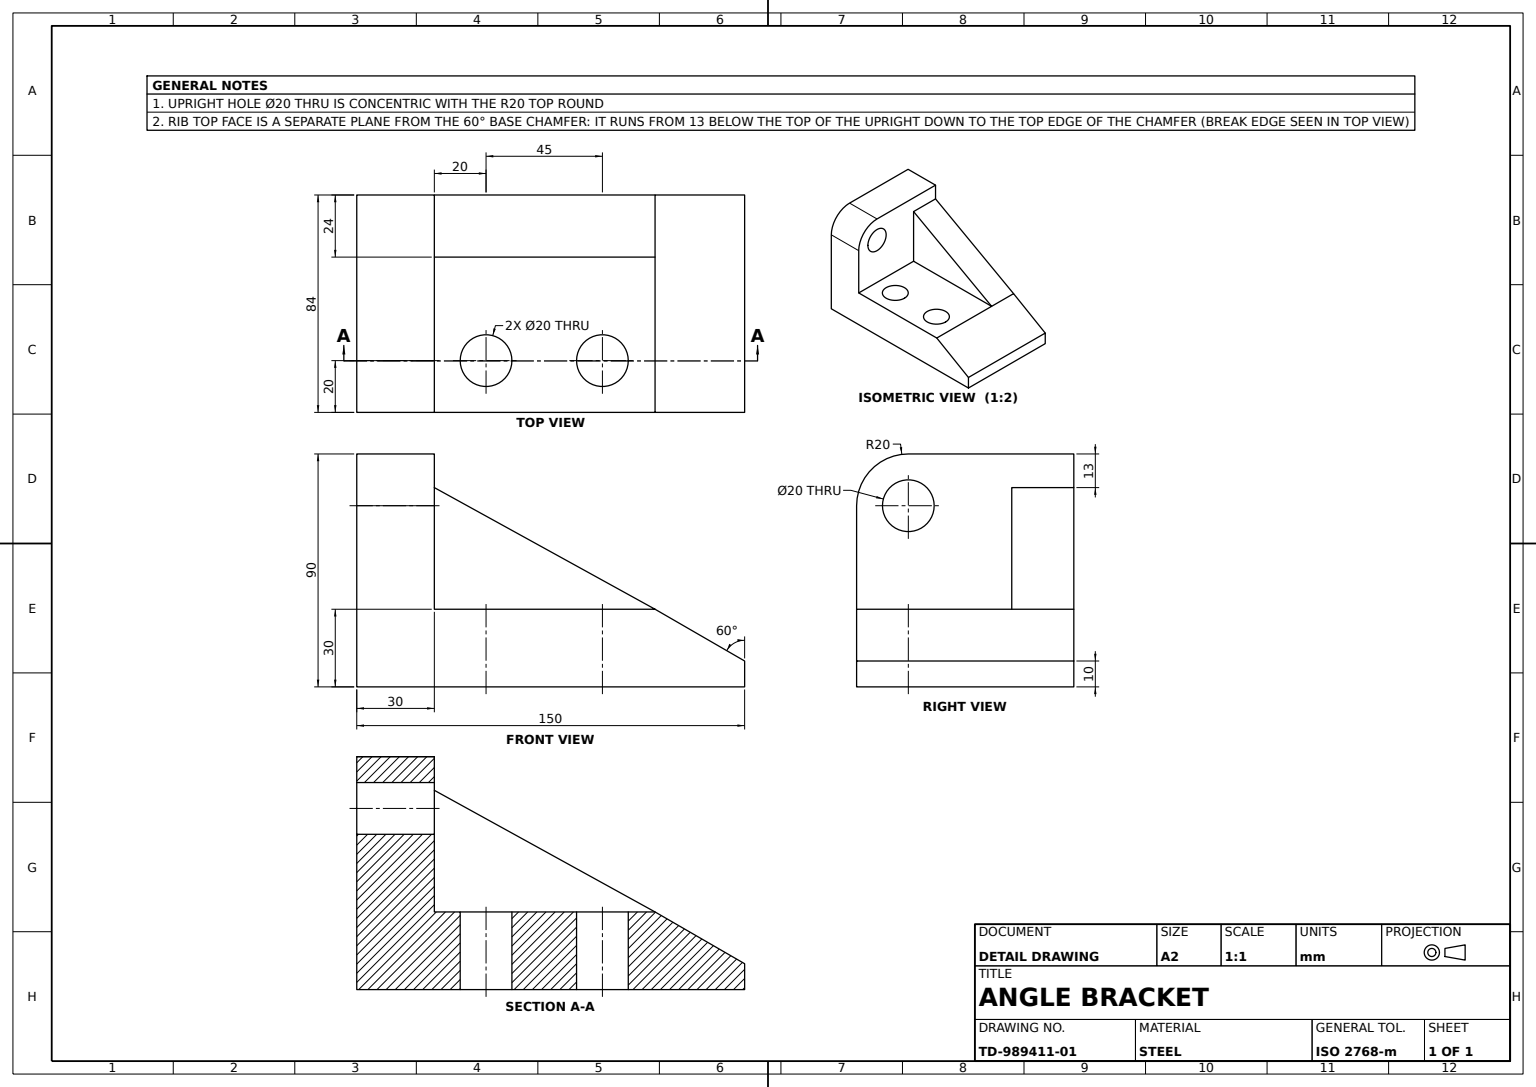
SolidWorks part; units mm, degrees
material "Plain Carbon Steel"
ref_plane "Front Plane" through (0, 0, 0) normal (0, 0, 1) x (1, 0, 0)
ref_plane "Top Plane" through (0, 0, 0) normal (0, 1, 0) x (1, 0, 0)
ref_plane "Right Plane" through (0, 0, 0) normal (1, 0, 0) x (0, 0, -1)
sketch "Bracket Profile Sketch" plane through (0, 0, 0) normal (0, 0, 1) x (1, 0, 0)
  line L0 (-75, 90) -> (-75, 0)
  line L1 (-75, 0) -> (75, 0)
  line L2 (75, 0) -> (75, 10)
  line L3 (75, 10) -> (40.359, 30)
  line L4 (40.359, 30) -> (-45, 30)
  line L5 (-45, 30) -> (-45, 90)
  line L6 (-45, 90) -> (-75, 90)
  dimension "D1" = 90
  dimension "D2" = 150
  dimension "D3" = 10
  dimension "D4" = 30
  dimension "D5" = 60
  dimension "D6" = 30
extrude "Bracket Body" add sketch "Bracket Profile Sketch" along normal mid plane 84
fillet "Upright Top Round R20" radius 20 1 edges at (-60, 90, 42)
sketch "Support Rib Sketch" plane through (0, 0, -42) normal (0, 0, -1) x (-1, 0, 0)
  line L0 (-40.359, 30) -> (45, 77)
  line L1 (45, 30) -> (45, 90) construction
  line L2 (45, 90) -> (75, 90) construction
  dimension "D1" = 13
rib "Support Rib" sketch "Support Rib Sketch" sketch "Support Rib Sketch" thickness 24 extrusion direction parallel to sketch draft on no parameters "D1"=24
sketch "Base Mounting Holes Sketch" plane through (0, 30, 0) normal (0, 1, 0) x (1, 0, 0)
  line L0 (40.359, -42) -> (-45, -42) construction
  line L1 (-45, -22) -> (-45, 42) construction
  circle A0 centre (-25, -22) radius 10
  circle A1 centre (20, -22) radius 10
  dimension "D1" = 20
  dimension "D2" = 45
  dimension "D3" = 20
  dimension "D4" = 20
extrude "Base Mounting Holes" cut sketch "Base Mounting Holes Sketch" against normal up to next
sketch "Upright Hole Sketch" plane through (-45, 0, 0) normal (1, 0, 0) x (0, 0, -1)
  circle A0 centre (-22, 70) radius 10
  dimension "D1" = 20
extrude "Upright Hole Ø20" cut sketch "Upright Hole Sketch" against normal up to next
